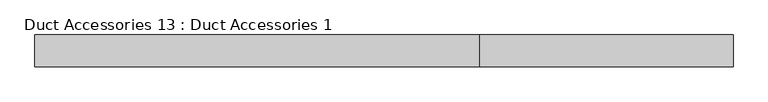
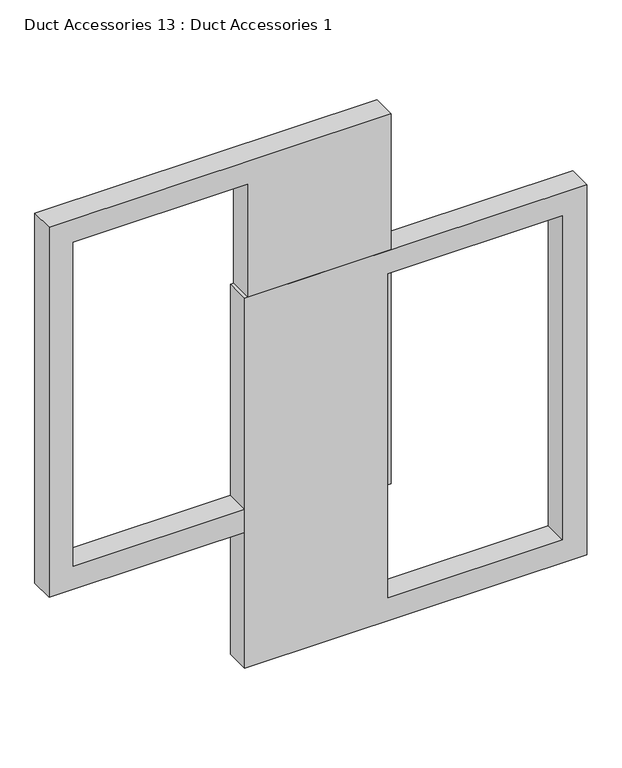
"""IFC4 building model written with IfcOpenShell, lengths in millimetres: damper geometry, Duct Accessories 13 : Duct Accessories 1."""

from ifc_helpers import new_model, si_unit, frame, origin, place, context, project, spatial, polyline, outline, extrude, source, transform, mapped, element, save


def duct_accessories_13_duct_accessories_1_4da7b8f5(model_context):
    return source(origin(), model_context, "Body", "SweptSolid", [
        extrude(outline(polyline([(1799.1403114, -12928.36893), (579.9403114, -12928.36893), (579.9403114, -11861.56893), (1799.1403114, -11861.56893), (1799.1403114, -12928.36893)]), holes=[polyline([(1722.9403114, -12480.9324751), (1722.9403114, -11937.76893), (656.1403114, -11937.76893), (656.1403114, -12480.9324751), (1722.9403114, -12480.9324751)])]), frame((0.0, -447.4934478, 0.0), z_axis=(0.0, 1.0, 0.0), x_axis=(0.0, 0.0, 1.0)), (0.0, 0.0, 1.0), 76.2),
        extrude(outline(polyline([(2246.5767663, -12471.5606701), (2246.5767663, -13538.3606701), (1027.3767663, -13538.3606701), (1027.3767663, -12471.5606701), (2246.5767663, -12471.5606701)]), holes=[polyline([(2170.3767663, -12918.997125), (1103.5767663, -12918.997125), (1103.5767663, -13462.1606701), (2170.3767663, -13462.1606701), (2170.3767663, -12918.997125)])]), frame((0.0, -447.4934478, 0.0), z_axis=(0.0, 1.0, 0.0), x_axis=(0.0, 0.0, 1.0)), (0.0, 0.0, 1.0), 76.2),
    ])


if __name__ == "__main__":
    model = new_model("IFC4")
    model_context = context("Model", 3, world=origin())
    ifc_project = project(units=[si_unit("LENGTHUNIT", "METRE", prefix="MILLI")], contexts=[model_context])
    site = spatial("IfcSite", under=ifc_project)
    building = spatial("IfcBuilding", under=site)
    placement = place(None, origin())
    duct_accessories_13_duct_accessories_1_shape = duct_accessories_13_duct_accessories_1_4da7b8f5(model_context)
    element("IfcDamper", 1, ObjectType="Duct Accessories 13 : Duct Accessories 1", at=placement, inside=building, context=model_context, shape_type="MappedRepresentation", body=[
        mapped(duct_accessories_13_duct_accessories_1_shape, transform((0.0, 0.0, 0.0), x_axis=(1.0, 0.0, 0.0), y_axis=(0.0, 1.0, 0.0), z_axis=(0.0, 0.0, 1.0))),
    ])
    save(model, "model.ifc")

# Revit data of these elements
# Element 1 (IfcDamper, "Duct Accessories 13 : Duct Accessories 1")
#   Materials on its faces: "border"
# Materials
#   "border": class "Generic", colour RGB 144 144 144, transparency 0, Cost = 0
